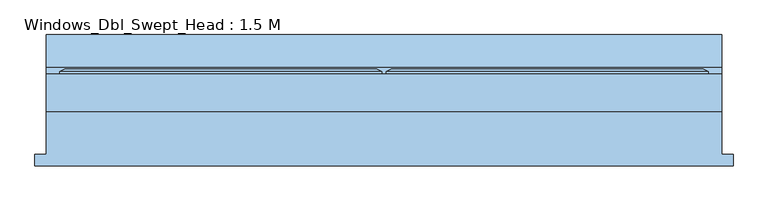
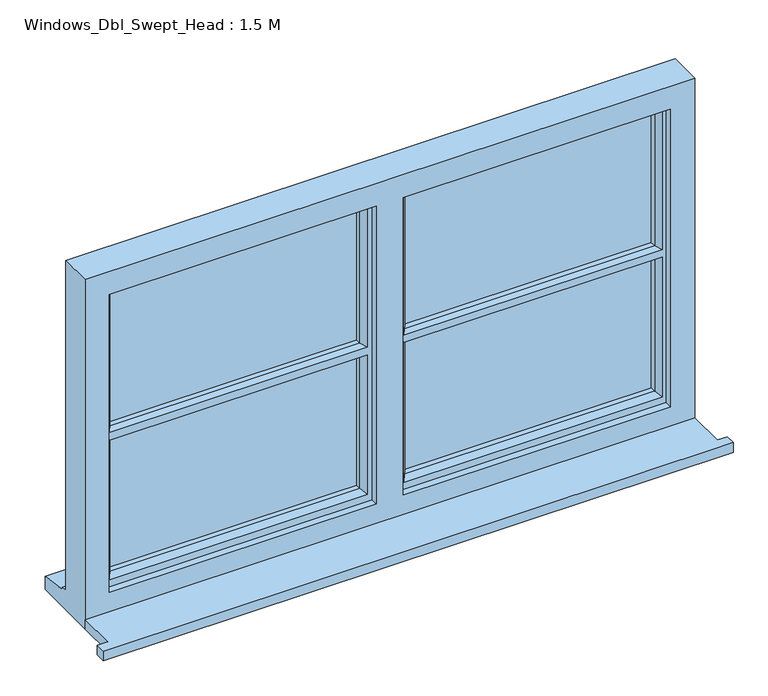
"""IFC4 building model written with IfcOpenShell, lengths in millimetres: window geometry, Windows_Dbl_Swept_Head : 1.5 M."""

from ifc_helpers import new_model, si_unit, frame, origin, place, context, project, spatial, polyline, circle_curve, outline, extrude, faceted_brep, source, transform, mapped, element, save
from ifc_brep_helpers import plane_surface, revolved_surface, advanced_brep


def windows_dbl_swept_head_1_5_m_7eee1f0c(model_context):
    return source(origin(), model_context, "Body", "SolidModel", [
        extrude(outline(polyline([(-1060.0, -130.8434322), (-1060.0, -105.8434322), (-1035.0, -105.8434322), (-1035.0, -10.2434322), (465.0, -10.2434322), (465.0, -105.8434322), (490.0, -105.8434322), (490.0, -130.8434322), (-1060.0, -130.8434322)])), frame((0.0, 0.0, 1200.0), z_axis=(0.0, 0.0, 1.0), x_axis=(1.0, 0.0, 0.0)), (0.0, 0.0, 1.0), 25.0),
        extrude(outline(polyline([(395.1480377, 36.7565678), (-240.0, 36.7565678), (-240.0, 60.7565678), (395.1480377, 60.7565678), (395.1480377, 36.7565678)])), frame((0.0, 0.0, 1293.0), z_axis=(0.0, 0.0, 1.0), x_axis=(1.0, 0.0, 0.0)), (0.0, 0.0, 1.0), 365.5),
        extrude(outline(polyline([(395.1480377, 36.7565678), (-240.0, 36.7565678), (-240.0, 60.7565678), (395.1480377, 60.7565678), (395.1480377, 36.7565678)])), frame((0.0, 0.0, 1674.5), z_axis=(0.0, 0.0, 1.0), x_axis=(1.0, 0.0, 0.0)), (0.0, 0.0, 1.0), 365.5),
        extrude(outline(polyline([(-330.0, 36.7565678), (-965.0, 36.7565678), (-965.0, 60.7565678), (-330.0, 60.7565678), (-330.0, 36.7565678)])), frame((0.0, 0.0, 1674.5), z_axis=(0.0, 0.0, 1.0), x_axis=(1.0, 0.0, 0.0)), (0.0, 0.0, 1.0), 365.5),
        extrude(outline(polyline([(-330.0, 36.7565678), (-965.1480377, 36.7565678), (-965.1480377, 60.7565678), (-330.0, 60.7565678), (-330.0, 36.7565678)])), frame((0.0, 0.0, 1292.8519623), z_axis=(0.0, 0.0, 1.0), x_axis=(1.0, 0.0, 0.0)), (0.0, 0.0, 1.0), 365.6480377),
        faceted_brep([(-1035.0, -10.2434322, 1200.0), (465.0, -10.2434322, 1200.0), (465.0, -10.2434322, 2110.0), (-1035.0, -10.2434322, 2110.0), (-318.0, -10.2434322, 2050.0), (-318.0, -10.2434322, 1275.0), (-975.0, -10.2434322, 1275.0), (-975.0, -10.2434322, 2050.0), (-252.0, -10.2434322, 2050.0), (405.0, -10.2434322, 2050.0), (405.0, -10.2434322, 1275.0), (-252.0, -10.2434322, 1275.0), (-1035.0, 72.7565678, 2110.0), (-1035.0, 72.7565678, 1251.0), (-1035.0, 87.7565678, 1249.68767), (-1035.0, 87.7565678, 1244.7449676), (-1035.0, 160.2565678, 1233.8088847), (-1035.0, 160.2565678, 1200.0), (465.0, 72.7565678, 2110.0), (465.0, 72.7565678, 1251.0), (-995.0, 72.7565678, 2070.0), (-995.0, 72.7565678, 1263.0), (-300.0, 72.7565678, 1263.0), (-300.0, 72.7565678, 2070.0), (-270.0, 72.7565678, 2070.0), (-270.0, 72.7565678, 1263.0), (425.0, 72.7565678, 1263.0), (425.0, 72.7565678, 2070.0), (-995.0, 7.7565678, 2070.0), (-995.0, 7.7565678, 1263.0), (-300.0, 7.7565678, 2070.0), (-300.0, 7.7565678, 1263.0), (-318.0, 7.7565678, 2050.0), (-975.0, 7.7565678, 2050.0), (-975.0, 7.7565678, 1275.0), (-318.0, 7.7565678, 1275.0), (-270.0, 7.7565678, 2070.0), (425.0, 7.7565678, 2070.0), (425.0, 7.7565678, 1263.0), (-270.0, 7.7565678, 1263.0), (405.0, 7.7565678, 2050.0), (-252.0, 7.7565678, 2050.0), (-252.0, 7.7565678, 1275.0), (405.0, 7.7565678, 1275.0), (465.0, 160.2565678, 1200.0), (465.0, 160.2565678, 1233.8088847), (465.0, 87.7565678, 1244.7449676), (465.0, 87.7565678, 1249.68767)], [[[0, 1, 2, 3], [4, 5, 6, 7], [8, 9, 10, 11]], [[0, 3, 12, 13, 14, 15, 16, 17]], [[13, 12, 18, 19], [20, 21, 22, 23], [24, 25, 26, 27]], [[21, 20, 28, 29]], [[28, 30, 31, 29], [32, 33, 34, 35]], [[36, 37, 38, 39], [40, 41, 42, 43]], [[33, 7, 6, 34]], [[12, 3, 2, 18]], [[28, 20, 23, 30]], [[27, 37, 36, 24]], [[7, 33, 32, 4]], [[40, 9, 8, 41]], [[19, 18, 2, 1, 44, 45, 46, 47]], [[27, 26, 38, 37]], [[9, 40, 43, 10]], [[23, 22, 31, 30]], [[25, 24, 36, 39]], [[41, 8, 11, 42]], [[4, 32, 35, 5]], [[44, 1, 0, 17]], [[45, 44, 17, 16]], [[46, 45, 16, 15]], [[47, 46, 15, 14]], [[19, 47, 14, 13]], [[22, 21, 29, 31]], [[26, 25, 39, 38]], [[11, 10, 43, 42]], [[35, 34, 6, 5]]]),
        advanced_brep(
        [(-280.0, 72.7565678, 2080.0), (-280.0, 78.5300705, 2080.0), (-280.0, 78.5300705, 1253.0), (-280.0, 72.7565678, 1253.0), (-270.0, 7.7565678, 2070.0), (-270.0, 72.7565678, 2070.0), (-270.0, 72.7565678, 1263.0), (-270.0, 7.7565678, 1263.0), (-230.0, 22.2494677, 2030.0), (-240.1480377, 7.7565678, 2040.1480377), (-240.1480377, 7.7565678, 1676.3519623), (-230.0, 22.2494677, 1681.5), (-240.1480377, 7.7565678, 1292.8519623), (-230.0, 22.2494677, 1303.0), (-230.0, 22.2494677, 1651.5), (-240.1480377, 7.7565678, 1656.6480377), (-230.0, 36.7565678, 2030.0), (-230.0, 36.7565678, 1681.5), (-230.0, 36.7565678, 1303.0), (-230.0, 36.7565678, 1651.5), (-240.0, 60.7565678, 2040.0), (-240.0, 36.7565678, 2040.0), (-240.0, 36.7565678, 1674.5), (-240.0, 60.7565678, 1674.5), (-240.0, 36.7565678, 1293.0), (-240.0, 60.7565678, 1293.0), (-240.0, 60.7565678, 1658.5), (-240.0, 36.7565678, 1658.5), (-230.0, 60.7565678, 1303.0), (-230.0, 78.5300705, 1303.0), (-230.0, 78.5300705, 1651.5), (-230.0, 60.7565678, 1651.5), (-230.0, 60.7565678, 1681.5), (-230.0, 78.5300705, 1681.5), (-230.0, 78.5300705, 1953.8431839), (-230.0, 60.7565678, 1953.8431839), (-247.4457548, 84.3035732, 2047.4457548), (-230.0, 78.5300705, 2030.0), (-235.0, 80.1847718, 1681.5), (-247.4457548, 84.3035732, 1669.0542452), (-247.4457548, 84.3035732, 1285.5542452), (-247.4457548, 84.3035732, 1663.9457548), (-235.0, 80.1847718, 1651.5), (-269.2153903, 84.3035732, 2069.2153903), (-269.2153903, 84.3035732, 1263.7846097), (435.0, 78.5300705, 1253.0), (435.0, 72.7565678, 1253.0), (425.0, 72.7565678, 1263.0), (425.0, 7.7565678, 1263.0), (395.1480377, 7.7565678, 1292.8519623), (385.0, 22.2494677, 1303.0), (385.0, 36.7565678, 1303.0), (395.0, 36.7565678, 1293.0), (395.0, 60.7565678, 1293.0), (385.0, 60.7565678, 1303.0), (385.0, 78.5300705, 1303.0), (402.4457548, 84.3035732, 1285.5542452), (424.2153903, 84.3035732, 1263.7846097), (435.0, 78.5300705, 2080.0), (435.0, 72.7565678, 2080.0), (425.0, 72.7565678, 2070.0), (425.0, 7.7565678, 2070.0), (395.1480377, 7.7565678, 1656.6480377), (385.0, 22.2494677, 1651.5), (395.1480377, 7.7565678, 2040.1480377), (385.0, 22.2494677, 2030.0), (385.0, 22.2494677, 1681.5), (395.1480377, 7.7565678, 1676.3519623), (385.0, 36.7565678, 1651.5), (385.0, 36.7565678, 2030.0), (385.0, 36.7565678, 1681.5), (395.0, 36.7565678, 1658.5), (395.0, 60.7565678, 1658.5), (395.0, 36.7565678, 2040.0), (395.0, 60.7565678, 2040.0), (395.0, 60.7565678, 1674.5), (395.0, 36.7565678, 1674.5), (385.0, 60.7565678, 1651.5), (385.0, 78.5300705, 1651.5), (385.0, 78.5300705, 1681.5), (385.0, 60.7565678, 1681.5), (385.0, 60.7565678, 1953.8431839), (385.0, 78.5300705, 1953.8431839), (390.0, 80.1847718, 1651.5), (402.4457548, 84.3035732, 1663.9457548), (385.0, 78.5300705, 2030.0), (402.4457548, 84.3035732, 2047.4457548), (402.4457548, 84.3035732, 1669.0542452), (390.0, 80.1847718, 1681.5), (424.2153903, 84.3035732, 2069.2153903)],
        [
            (0, 1),
            (1, 2),
            (2, 3),
            (3, 0),
            (4, 5),
            (5, 6),
            (6, 7),
            (7, 4),
            (8, 9),
            (9, 10),
            (10, 11),
            (11, 8),
            (12, 13),
            (13, 14),
            (14, 15),
            (15, 12),
            (16, 8),
            (11, 17),
            (17, 16),
            (13, 18),
            (18, 19),
            (19, 14),
            (20, 21),
            (21, 22),
            (22, 23),
            (23, 20),
            (24, 25),
            (25, 26),
            (26, 27),
            (27, 24),
            (28, 29),
            (29, 30),
            (30, 31),
            (31, 28),
            (32, 33),
            (33, 34),
            (34, 35),
            (35, 32),
            (36, 37),
            (37, 34),
            (33, 38),
            (38, 39),
            (39, 36),
            (29, 40),
            (40, 41),
            (41, 42),
            (42, 30),
            (1, 43),
            (43, 44),
            (44, 2),
            (2, 45),
            (45, 46),
            (46, 3),
            (6, 47),
            (47, 48),
            (48, 7),
            (12, 49),
            (49, 50),
            (50, 13),
            (50, 51),
            (51, 18),
            (24, 52),
            (52, 53),
            (53, 25),
            (28, 54),
            (54, 55),
            (55, 29),
            (55, 56),
            (56, 40),
            (44, 57),
            (57, 45),
            (45, 58),
            (58, 59),
            (59, 46),
            (47, 60),
            (60, 61),
            (61, 48),
            (49, 62),
            (62, 63),
            (63, 50),
            (64, 65),
            (65, 66),
            (66, 67),
            (67, 64),
            (63, 68),
            (68, 51),
            (65, 69),
            (69, 70),
            (70, 66),
            (52, 71),
            (71, 72),
            (72, 53),
            (73, 74),
            (74, 75),
            (75, 76),
            (76, 73),
            (54, 77),
            (77, 78),
            (78, 55),
            (79, 80),
            (80, 81),
            (81, 82),
            (82, 79),
            (78, 83),
            (83, 84),
            (84, 56),
            (85, 86),
            (86, 87),
            (87, 88),
            (88, 79),
            (82, 85),
            (57, 89),
            (89, 58),
            (0, 59),
            (58, 1),
            (5, 60),
            (4, 61),
            (15, 62),
            (9, 64),
            (67, 10),
            (8, 65),
            (16, 69),
            (27, 71),
            (68, 19),
            (21, 73),
            (76, 22),
            (17, 70),
            (20, 74),
            (72, 26),
            (31, 77),
            (23, 75),
            (80, 32),
            (35, 81, circle_curve(frame((77.5, 60.7565678, 1325.0), z_axis=(0.0, 1.0, 0.0), x_axis=(1.0, 0.0, 0.0)), 700.0)),
            (36, 86),
            (85, 37),
            (43, 89),
            (84, 41),
            (39, 87),
            (38, 88),
            (11, 66),
            (14, 63),
            (42, 83),
            (82, 34, circle_curve(frame((77.5, 78.5300705, 1325.0), z_axis=(0.0, -1.0, 0.0), x_axis=(1.0, 0.0, 0.0)), 700.0)),
        ],
        [
            plane_surface(frame((-280.0, 78.5300705, 2080.0), z_axis=(-1.0, 0.0, 0.0), x_axis=(0.0, 0.0, -1.0))),
            plane_surface(frame((-270.0, 72.7565678, 2070.0), z_axis=(-1.0, 0.0, 0.0), x_axis=(0.0, 0.0, -1.0))),
            plane_surface(frame((-240.1480377, 7.7565678, 2040.1480377), z_axis=(0.8191520442889492, -0.5735764363511071, 0.0), x_axis=(0.0, 0.0, -1.0))),
            plane_surface(frame((-230.0, 22.2494677, 2030.0), z_axis=(1.0, 0.0, 0.0), x_axis=(0.0, 0.0, -1.0))),
            plane_surface(frame((-240.0, 36.7565678, 2040.0), z_axis=(1.0, 0.0, 0.0), x_axis=(0.0, 0.0, -1.0))),
            plane_surface(frame((-230.0, 60.7565678, 2030.0), z_axis=(1.0, 0.0, 0.0), x_axis=(0.0, 0.0, -1.0))),
            plane_surface(frame((-230.0, 78.5300705, 2030.0), z_axis=(0.31418232948755237, 0.9493626619147053, 0.0), x_axis=(0.0, 0.0, -1.0))),
            plane_surface(frame((-269.2153903, 84.3035732, 2069.2153903), z_axis=(-0.47196942945730275, 0.8816149146071363, 0.0), x_axis=(0.0, 0.0, -1.0))),
            plane_surface(frame((-280.0, 78.5300705, 1253.0), z_axis=(0.0, 0.0, -1.0), x_axis=(1.0, 0.0, 0.0))),
            plane_surface(frame((-270.0, 72.7565678, 1263.0), z_axis=(0.0, 0.0, -1.0), x_axis=(1.0, 0.0, 0.0))),
            plane_surface(frame((-240.1480377, 7.7565678, 1292.8519623), z_axis=(0.0, -0.5735764363511044, 0.819152044288951), x_axis=(1.0, 0.0, 0.0))),
            plane_surface(frame((-230.0, 22.2494677, 1303.0), z_axis=(0.0, 0.0, 1.0), x_axis=(1.0, 0.0, 0.0))),
            plane_surface(frame((-240.0, 36.7565678, 1293.0), z_axis=(0.0, 0.0, 1.0), x_axis=(1.0, 0.0, 0.0))),
            plane_surface(frame((-230.0, 60.7565678, 1303.0), z_axis=(0.0, 0.0, 1.0), x_axis=(1.0, 0.0, 0.0))),
            plane_surface(frame((-230.0, 78.5300705, 1303.0), z_axis=(0.0, 0.9493626619147063, 0.31418232948754926), x_axis=(1.0, 0.0, 0.0))),
            plane_surface(frame((-269.2153903, 84.3035732, 1263.7846097), z_axis=(0.0, 0.8816149146071347, -0.47196942945730563), x_axis=(1.0, 0.0, 0.0))),
            plane_surface(frame((435.0, 78.5300705, 1253.0), z_axis=(1.0, 0.0, 0.0), x_axis=(0.0, 0.0, 1.0))),
            plane_surface(frame((425.0, 72.7565678, 1263.0), z_axis=(1.0, 0.0, 0.0), x_axis=(0.0, 0.0, 1.0))),
            plane_surface(frame((395.1480377, 7.7565678, 1292.8519623), z_axis=(-0.8191520442889529, -0.5735764363511018, 0.0), x_axis=(0.0, 0.0, 1.0))),
            plane_surface(frame((385.0, 22.2494677, 1303.0), z_axis=(-1.0, 0.0, 0.0), x_axis=(0.0, 0.0, 1.0))),
            plane_surface(frame((395.0, 36.7565678, 1293.0), z_axis=(-1.0, 0.0, 0.0), x_axis=(0.0, 0.0, 1.0))),
            plane_surface(frame((385.0, 60.7565678, 1303.0), z_axis=(-1.0, 0.0, 0.0), x_axis=(0.0, 0.0, 1.0))),
            plane_surface(frame((385.0, 78.5300705, 1303.0), z_axis=(-0.3141823294875462, 0.9493626619147074, 0.0), x_axis=(0.0, 0.0, 1.0))),
            plane_surface(frame((424.2153903, 84.3035732, 1263.7846097), z_axis=(0.4719694294573085, 0.8816149146071331, 0.0), x_axis=(0.0, 0.0, 1.0))),
            plane_surface(frame((435.0, 78.5300705, 2080.0), z_axis=(0.0, 0.0, 1.0), x_axis=(-1.0, 0.0, 0.0))),
            plane_surface(frame((435.0, 72.7565678, 2080.0), z_axis=(0.0, -1.0, 0.0), x_axis=(-1.0, 0.0, 0.0))),
            plane_surface(frame((425.0, 72.7565678, 2070.0), z_axis=(0.0, 0.0, 1.0), x_axis=(-1.0, 0.0, 0.0))),
            plane_surface(frame((425.0, 7.7565678, 2070.0), z_axis=(0.0, -1.0, 0.0), x_axis=(-1.0, 0.0, 0.0))),
            plane_surface(frame((395.1480377, 7.7565678, 2040.1480377), z_axis=(0.0, -0.5735764363511044, -0.819152044288951), x_axis=(-1.0, 0.0, 0.0))),
            plane_surface(frame((385.0, 22.2494677, 2030.0), z_axis=(0.0, 0.0, -1.0), x_axis=(-1.0, 0.0, 0.0))),
            plane_surface(frame((385.0, 36.7565678, 2030.0), z_axis=(0.0, 1.0, 0.0), x_axis=(-1.0, 0.0, 0.0))),
            plane_surface(frame((395.0, 36.7565678, 2040.0), z_axis=(0.0, 0.0, -1.0), x_axis=(-1.0, 0.0, 0.0))),
            plane_surface(frame((395.0, 60.7565678, 2040.0), z_axis=(0.0, -1.0, 0.0), x_axis=(-1.0, 0.0, 0.0))),
            plane_surface(frame((385.0, 78.5300705, 2030.0), z_axis=(0.0, 0.9493626619147064, -0.3141823294875493), x_axis=(-1.0, 0.0, 0.0))),
            plane_surface(frame((402.4457548, 84.3035732, 2047.4457548), z_axis=(0.0, 1.0, 0.0), x_axis=(-1.0, 0.0, 0.0))),
            plane_surface(frame((424.2153903, 84.3035732, 2069.2153903), z_axis=(0.0, 0.8816149146071347, 0.47196942945730563), x_axis=(-1.0, 0.0, 0.0))),
            plane_surface(frame((402.4457548, 84.3035732, 1669.0542452), z_axis=(0.0, 0.9493626619145938, 0.3141823294878896), x_axis=(-1.0, 0.0, 0.0))),
            plane_surface(frame((402.4457548, 80.1847718, 1681.5), z_axis=(0.0, 0.0, 1.0), x_axis=(-1.0, 0.0, 0.0))),
            plane_surface(frame((402.4457548, 60.7565678, 1674.5), z_axis=(0.0, 0.0, 1.0), x_axis=(-1.0, 0.0, 0.0))),
            plane_surface(frame((402.4457548, 36.7565678, 1681.5), z_axis=(0.0, 0.0, 1.0), x_axis=(-1.0, 0.0, 0.0))),
            plane_surface(frame((402.4457548, 22.2494677, 1681.5), z_axis=(0.0, -0.33472142672711697, 0.9423171262848634), x_axis=(-1.0, 0.0, 0.0))),
            plane_surface(frame((402.4457548, 7.7565678, 1656.6480377), z_axis=(0.0, -0.33472142672499106, -0.9423171262856186), x_axis=(-1.0, 0.0, 0.0))),
            plane_surface(frame((402.4457548, 22.2494677, 1651.5), z_axis=(0.0, 0.0, -1.0), x_axis=(-1.0, 0.0, 0.0))),
            plane_surface(frame((402.4457548, 36.7565678, 1658.5), z_axis=(0.0, 0.0, -1.0), x_axis=(-1.0, 0.0, 0.0))),
            plane_surface(frame((402.4457548, 60.7565678, 1651.5), z_axis=(0.0, 0.0, -1.0), x_axis=(-1.0, 0.0, 0.0))),
            plane_surface(frame((402.4457548, 80.1847718, 1651.5), z_axis=(0.0, 0.9493626619148547, -0.31418232948710106), x_axis=(-1.0, 0.0, 0.0))),
            plane_surface(frame((-230.0, 78.5300705, 2030.0), z_axis=(0.0, 1.0, 0.0), x_axis=(0.0, 0.0, 1.0))),
            revolved_surface(polyline([(777.5, 78.5300705, 1325.0), (777.5, 60.7565678, 1325.0)]), (77.5, 78.5300705, 1325.0), (0.0, 1.0, 0.0)),
        ],
        [
            (0, [[1, 2, 3, 4]]),
            (1, [[5, 6, 7, 8]]),
            (2, [[9, 10, 11, 12]]),
            (2, [[13, 14, 15, 16]]),
            (3, [[17, -12, 18, 19]]),
            (3, [[20, 21, 22, -14]]),
            (4, [[23, 24, 25, 26]]),
            (4, [[27, 28, 29, 30]]),
            (5, [[31, 32, 33, 34]]),
            (5, [[35, 36, 37, 38]]),
            (6, [[39, 40, -36, 41, 42, 43]]),
            (6, [[44, 45, 46, 47, -32]]),
            (7, [[-2, 48, 49, 50]]),
            (8, [[-3, 51, 52, 53]]),
            (9, [[-7, 54, 55, 56]]),
            (10, [[-13, 57, 58, 59]]),
            (11, [[-20, -59, 60, 61]]),
            (12, [[-27, 62, 63, 64]]),
            (13, [[-31, 65, 66, 67]]),
            (14, [[-44, -67, 68, 69]]),
            (15, [[-50, 70, 71, -51]]),
            (16, [[-52, 72, 73, 74]]),
            (17, [[-55, 75, 76, 77]]),
            (18, [[-58, 78, 79, 80]]),
            (18, [[81, 82, 83, 84]]),
            (19, [[-60, -80, 85, 86]]),
            (19, [[87, 88, 89, -82]]),
            (20, [[-63, 90, 91, 92]]),
            (20, [[93, 94, 95, 96]]),
            (21, [[-66, 97, 98, 99]]),
            (21, [[100, 101, 102, 103]]),
            (22, [[-68, -99, 104, 105, 106]]),
            (22, [[107, 108, 109, 110, -103, 111]]),
            (23, [[-71, 112, 113, -72]]),
            (24, [[-1, 114, -73, 115]]),
            (25, [[-4, -53, -74, -114], [-6, 116, -75, -54]]),
            (26, [[-5, 117, -76, -116]]),
            (27, [[-8, -56, -77, -117], [-57, -16, 118, -78], [119, -84, 120, -10]]),
            (28, [[-9, 121, -81, -119]]),
            (29, [[-17, 122, -87, -121]]),
            (30, [[-62, -30, 123, -90], [-61, -86, 124, -21]]),
            (30, [[125, -96, 126, -24], [-122, -19, 127, -88]]),
            (31, [[-23, 128, -93, -125]]),
            (32, [[-64, -92, 129, -28], [-65, -34, 130, -97]]),
            (32, [[-128, -26, 131, -94], [132, -38, 133, -101]]),
            (33, [[-39, 134, -107, 135]]),
            (34, [[-49, 136, -112, -70], [-69, -106, 137, -45], [-134, -43, 138, -108]]),
            (35, [[-48, -115, -113, -136]]),
            (36, [[-138, -42, 139, -109]]),
            (37, [[-132, -100, -110, -139, -41, -35]]),
            (38, [[-25, -126, -95, -131]]),
            (39, [[140, -89, -127, -18]]),
            (40, [[-120, -83, -140, -11]]),
            (41, [[-118, -15, 141, -79]]),
            (42, [[-141, -22, -124, -85]]),
            (43, [[-29, -129, -91, -123]]),
            (44, [[-130, -33, -47, 142, -104, -98]]),
            (45, [[-137, -105, -142, -46]]),
            (46, [[143, -40, -135, -111]]),
            (47, [[-133, -37, -143, -102]]),
        ],
    ),
        advanced_brep(
        [(-330.0, 60.7565678, 2040.0), (-965.0, 60.7565678, 2040.0), (-965.0, 60.7565678, 1674.5), (-330.0, 60.7565678, 1674.5), (-955.0, 60.7565678, 1953.8431839), (-340.0, 60.7565678, 1953.8431839), (-340.0, 60.7565678, 1681.5), (-955.0, 60.7565678, 1681.5), (-965.0, 60.7565678, 1293.0), (-330.0, 60.7565678, 1293.0), (-330.0, 60.7565678, 1658.5), (-965.0, 60.7565678, 1658.5), (-340.0, 60.7565678, 1303.0), (-955.0, 60.7565678, 1303.0), (-955.0, 60.7565678, 1651.5), (-340.0, 60.7565678, 1651.5), (-1005.0, 72.7565678, 2080.0), (-1005.0, 78.5300705, 2080.0), (-1005.0, 78.5300705, 1253.0), (-1005.0, 72.7565678, 1253.0), (-995.0, 7.7565678, 2070.0), (-995.0, 72.7565678, 2070.0), (-995.0, 72.7565678, 1263.0), (-995.0, 7.7565678, 1263.0), (-955.0, 22.2494677, 2030.0), (-965.1480377, 7.7565678, 2040.1480377), (-965.1480377, 7.7565678, 1676.3519623), (-955.0, 22.2494677, 1681.5), (-965.1480377, 7.7565678, 1292.8519623), (-955.0, 22.2494677, 1303.0), (-955.0, 22.2494677, 1651.5), (-965.1480377, 7.7565678, 1656.6480377), (-955.0, 36.7565678, 2030.0), (-955.0, 36.7565678, 1681.5), (-955.0, 36.7565678, 1303.0), (-955.0, 36.7565678, 1651.5), (-965.0, 36.7565678, 2040.0), (-965.0, 36.7565678, 1674.5), (-965.0, 36.7565678, 1293.0), (-965.0, 36.7565678, 1658.5), (-955.0, 78.5300705, 1303.0), (-955.0, 78.5300705, 1651.5), (-955.0, 78.5300705, 1681.5), (-955.0, 78.5300705, 1953.8431839), (-972.4457548, 84.3035732, 2047.4457548), (-955.0, 78.5300705, 2030.0), (-960.0, 80.1847718, 1681.5), (-972.4457548, 84.3035732, 1669.0542452), (-972.4457548, 84.3035732, 1285.5542452), (-972.4457548, 84.3035732, 1663.9457548), (-960.0, 80.1847718, 1651.5), (-994.2153903, 84.3035732, 2069.2153903), (-994.2153903, 84.3035732, 1263.7846097), (-290.0, 78.5300705, 1253.0), (-290.0, 72.7565678, 1253.0), (-300.0, 72.7565678, 1263.0), (-300.0, 7.7565678, 1263.0), (-329.8519623, 7.7565678, 1292.8519623), (-340.0, 22.2494677, 1303.0), (-340.0, 36.7565678, 1303.0), (-330.0, 36.7565678, 1293.0), (-340.0, 78.5300705, 1303.0), (-322.5542452, 84.3035732, 1285.5542452), (-300.7846097, 84.3035732, 1263.7846097), (-290.0, 78.5300705, 2080.0), (-290.0, 72.7565678, 2080.0), (-300.0, 72.7565678, 2070.0), (-300.0, 7.7565678, 2070.0), (-329.8519623, 7.7565678, 1656.6480377), (-340.0, 22.2494677, 1651.5), (-329.8519623, 7.7565678, 2040.1480377), (-340.0, 22.2494677, 2030.0), (-340.0, 22.2494677, 1681.5), (-329.8519623, 7.7565678, 1676.3519623), (-340.0, 36.7565678, 1651.5), (-340.0, 36.7565678, 2030.0), (-340.0, 36.7565678, 1681.5), (-330.0, 36.7565678, 1658.5), (-330.0, 36.7565678, 2040.0), (-330.0, 36.7565678, 1674.5), (-340.0, 78.5300705, 1651.5), (-340.0, 78.5300705, 1681.5), (-340.0, 78.5300705, 1953.8431839), (-335.0, 80.1847718, 1651.5), (-322.5542452, 84.3035732, 1663.9457548), (-340.0, 78.5300705, 2030.0), (-322.5542452, 84.3035732, 2047.4457548), (-322.5542452, 84.3035732, 1669.0542452), (-335.0, 80.1847718, 1681.5), (-300.7846097, 84.3035732, 2069.2153903)],
        [
            (0, 1),
            (1, 2),
            (2, 3),
            (3, 0),
            (4, 5, circle_curve(frame((-647.5, 60.7565678, 1325.0), z_axis=(0.0, 1.0, 0.0), x_axis=(1.0, 0.0, 0.0)), 700.0)),
            (5, 6),
            (6, 7),
            (7, 4),
            (8, 9),
            (9, 10),
            (10, 11),
            (11, 8),
            (12, 13),
            (13, 14),
            (14, 15),
            (15, 12),
            (16, 17),
            (17, 18),
            (18, 19),
            (19, 16),
            (20, 21),
            (21, 22),
            (22, 23),
            (23, 20),
            (24, 25),
            (25, 26),
            (26, 27),
            (27, 24),
            (28, 29),
            (29, 30),
            (30, 31),
            (31, 28),
            (32, 24),
            (27, 33),
            (33, 32),
            (29, 34),
            (34, 35),
            (35, 30),
            (1, 36),
            (36, 37),
            (37, 2),
            (38, 8),
            (11, 39),
            (39, 38),
            (13, 40),
            (40, 41),
            (41, 14),
            (7, 42),
            (42, 43),
            (43, 4),
            (44, 45),
            (45, 43),
            (42, 46),
            (46, 47),
            (47, 44),
            (40, 48),
            (48, 49),
            (49, 50),
            (50, 41),
            (17, 51),
            (51, 52),
            (52, 18),
            (18, 53),
            (53, 54),
            (54, 19),
            (22, 55),
            (55, 56),
            (56, 23),
            (28, 57),
            (57, 58),
            (58, 29),
            (58, 59),
            (59, 34),
            (38, 60),
            (60, 9),
            (12, 61),
            (61, 40),
            (61, 62),
            (62, 48),
            (52, 63),
            (63, 53),
            (53, 64),
            (64, 65),
            (65, 54),
            (55, 66),
            (66, 67),
            (67, 56),
            (57, 68),
            (68, 69),
            (69, 58),
            (70, 71),
            (71, 72),
            (72, 73),
            (73, 70),
            (69, 74),
            (74, 59),
            (71, 75),
            (75, 76),
            (76, 72),
            (60, 77),
            (77, 10),
            (78, 0),
            (3, 79),
            (79, 78),
            (15, 80),
            (80, 61),
            (81, 6),
            (5, 82),
            (82, 81),
            (80, 83),
            (83, 84),
            (84, 62),
            (85, 86),
            (86, 87),
            (87, 88),
            (88, 81),
            (82, 85),
            (63, 89),
            (89, 64),
            (16, 65),
            (64, 17),
            (21, 66),
            (20, 67),
            (31, 68),
            (25, 70),
            (73, 26),
            (24, 71),
            (32, 75),
            (39, 77),
            (74, 35),
            (36, 78),
            (79, 37),
            (33, 76),
            (44, 86),
            (85, 45),
            (51, 89),
            (84, 49),
            (47, 87),
            (46, 88),
            (83, 50),
            (69, 30),
            (72, 27),
            (82, 43, circle_curve(frame((-647.5, 78.5300705, 1325.0), z_axis=(0.0, -1.0, 0.0), x_axis=(1.0, 0.0, 0.0)), 700.0)),
        ],
        [
            plane_surface(frame((395.0, 60.7565678, 2040.0), z_axis=(0.0, -1.0, 0.0), x_axis=(-1.0, 0.0, 0.0))),
            plane_surface(frame((-1005.0, 78.5300705, 2080.0), z_axis=(-1.0, 0.0, 0.0), x_axis=(0.0, 0.0, -1.0))),
            plane_surface(frame((-995.0, 72.7565678, 2070.0), z_axis=(-1.0, 0.0, 0.0), x_axis=(0.0, 0.0, -1.0))),
            plane_surface(frame((-965.1480377, 7.7565678, 2040.1480377), z_axis=(0.8191520442889492, -0.5735764363511071, 0.0), x_axis=(0.0, 0.0, -1.0))),
            plane_surface(frame((-955.0, 22.2494677, 2030.0), z_axis=(1.0, 0.0, 0.0), x_axis=(0.0, 0.0, -1.0))),
            plane_surface(frame((-965.0, 36.7565678, 2040.0), z_axis=(1.0, 0.0, 0.0), x_axis=(0.0, 0.0, -1.0))),
            plane_surface(frame((-955.0, 60.7565678, 2030.0), z_axis=(1.0, 0.0, 0.0), x_axis=(0.0, 0.0, -1.0))),
            plane_surface(frame((-955.0, 78.5300705, 2030.0), z_axis=(0.31418232948755237, 0.9493626619147053, 0.0), x_axis=(0.0, 0.0, -1.0))),
            plane_surface(frame((-994.2153903, 84.3035732, 2069.2153903), z_axis=(-0.47196942945730275, 0.8816149146071363, 0.0), x_axis=(0.0, 0.0, -1.0))),
            plane_surface(frame((-1005.0, 78.5300705, 1253.0), z_axis=(0.0, 0.0, -1.0), x_axis=(1.0, 0.0, 0.0))),
            plane_surface(frame((-995.0, 72.7565678, 1263.0), z_axis=(0.0, 0.0, -1.0), x_axis=(1.0, 0.0, 0.0))),
            plane_surface(frame((-965.1480377, 7.7565678, 1292.8519623), z_axis=(0.0, -0.5735764363511044, 0.819152044288951), x_axis=(1.0, 0.0, 0.0))),
            plane_surface(frame((-955.0, 22.2494677, 1303.0), z_axis=(0.0, 0.0, 1.0), x_axis=(1.0, 0.0, 0.0))),
            plane_surface(frame((-965.0, 36.7565678, 1293.0), z_axis=(0.0, 0.0, 1.0), x_axis=(1.0, 0.0, 0.0))),
            plane_surface(frame((-955.0, 60.7565678, 1303.0), z_axis=(0.0, 0.0, 1.0), x_axis=(1.0, 0.0, 0.0))),
            plane_surface(frame((-955.0, 78.5300705, 1303.0), z_axis=(0.0, 0.9493626619147063, 0.31418232948754926), x_axis=(1.0, 0.0, 0.0))),
            plane_surface(frame((-994.2153903, 84.3035732, 1263.7846097), z_axis=(0.0, 0.8816149146071347, -0.47196942945730563), x_axis=(1.0, 0.0, 0.0))),
            plane_surface(frame((-290.0, 78.5300705, 1253.0), z_axis=(1.0, 0.0, 0.0), x_axis=(0.0, 0.0, 1.0))),
            plane_surface(frame((-300.0, 72.7565678, 1263.0), z_axis=(1.0, 0.0, 0.0), x_axis=(0.0, 0.0, 1.0))),
            plane_surface(frame((-329.8519623, 7.7565678, 1292.8519623), z_axis=(-0.8191520442889529, -0.5735764363511018, 0.0), x_axis=(0.0, 0.0, 1.0))),
            plane_surface(frame((-340.0, 22.2494677, 1303.0), z_axis=(-1.0, 0.0, 0.0), x_axis=(0.0, 0.0, 1.0))),
            plane_surface(frame((-330.0, 36.7565678, 1293.0), z_axis=(-1.0, 0.0, 0.0), x_axis=(0.0, 0.0, 1.0))),
            plane_surface(frame((-340.0, 60.7565678, 1303.0), z_axis=(-1.0, 0.0, 0.0), x_axis=(0.0, 0.0, 1.0))),
            plane_surface(frame((-340.0, 78.5300705, 1303.0), z_axis=(-0.3141823294875462, 0.9493626619147074, 0.0), x_axis=(0.0, 0.0, 1.0))),
            plane_surface(frame((-300.7846097, 84.3035732, 1263.7846097), z_axis=(0.4719694294573085, 0.8816149146071331, 0.0), x_axis=(0.0, 0.0, 1.0))),
            plane_surface(frame((-290.0, 78.5300705, 2080.0), z_axis=(0.0, 0.0, 1.0), x_axis=(-1.0, 0.0, 0.0))),
            plane_surface(frame((-290.0, 72.7565678, 2080.0), z_axis=(0.0, -1.0, 0.0), x_axis=(-1.0, 0.0, 0.0))),
            plane_surface(frame((-300.0, 72.7565678, 2070.0), z_axis=(0.0, 0.0, 1.0), x_axis=(-1.0, 0.0, 0.0))),
            plane_surface(frame((-300.0, 7.7565678, 2070.0), z_axis=(0.0, -1.0, 0.0), x_axis=(-1.0, 0.0, 0.0))),
            plane_surface(frame((-329.8519623, 7.7565678, 2040.1480377), z_axis=(0.0, -0.5735764363511044, -0.819152044288951), x_axis=(-1.0, 0.0, 0.0))),
            plane_surface(frame((-340.0, 22.2494677, 2030.0), z_axis=(0.0, 0.0, -1.0), x_axis=(-1.0, 0.0, 0.0))),
            plane_surface(frame((-340.0, 36.7565678, 2030.0), z_axis=(0.0, 1.0, 0.0), x_axis=(-1.0, 0.0, 0.0))),
            plane_surface(frame((-330.0, 36.7565678, 2040.0), z_axis=(0.0, 0.0, -1.0), x_axis=(-1.0, 0.0, 0.0))),
            plane_surface(frame((-340.0, 78.5300705, 2030.0), z_axis=(0.0, 0.9493626619147064, -0.3141823294875493), x_axis=(-1.0, 0.0, 0.0))),
            plane_surface(frame((-322.5542452, 84.3035732, 2047.4457548), z_axis=(0.0, 1.0, 0.0), x_axis=(-1.0, 0.0, 0.0))),
            plane_surface(frame((-300.7846097, 84.3035732, 2069.2153903), z_axis=(0.0, 0.8816149146071347, 0.47196942945730563), x_axis=(-1.0, 0.0, 0.0))),
            plane_surface(frame((-972.4457548, 80.1847718, 1681.5), z_axis=(0.0, 0.9493626619144715, 0.31418232948825914), x_axis=(1.0, 0.0, 0.0))),
            plane_surface(frame((-972.4457548, 84.3035732, 1663.9457548), z_axis=(0.0, 0.949362661914977, -0.3141823294867314), x_axis=(1.0, 0.0, 0.0))),
            plane_surface(frame((-972.4457548, 80.1847718, 1651.5), z_axis=(0.0, 0.0, -1.0), x_axis=(1.0, 0.0, 0.0))),
            plane_surface(frame((-972.4457548, 60.7565678, 1658.5), z_axis=(0.0, 0.0, -1.0), x_axis=(1.0, 0.0, 0.0))),
            plane_surface(frame((-972.4457548, 36.7565678, 1651.5), z_axis=(0.0, 0.0, -1.0), x_axis=(1.0, 0.0, 0.0))),
            plane_surface(frame((-972.4457548, 22.2494677, 1651.5), z_axis=(0.0, -0.3347214267259168, -0.9423171262852897), x_axis=(1.0, 0.0, 0.0))),
            plane_surface(frame((-972.4457548, 7.7565678, 1676.3519623), z_axis=(0.0, -0.33472142672616695, 0.9423171262852009), x_axis=(1.0, 0.0, 0.0))),
            plane_surface(frame((-972.4457548, 22.2494677, 1681.5), z_axis=(0.0, 0.0, 1.0), x_axis=(1.0, 0.0, 0.0))),
            plane_surface(frame((-972.4457548, 36.7565678, 1674.5), z_axis=(0.0, 0.0, 1.0), x_axis=(1.0, 0.0, 0.0))),
            plane_surface(frame((-972.4457548, 60.7565678, 1681.5), z_axis=(0.0, 0.0, 1.0), x_axis=(1.0, 0.0, 0.0))),
            plane_surface(frame((-230.0, 78.5300705, 2030.0), z_axis=(0.0, 1.0, 0.0), x_axis=(0.0, 0.0, 1.0))),
            revolved_surface(polyline([(52.5, 78.5300705, 1325.0), (52.5, 60.7565678, 1325.0)]), (-647.5, 72.7565678, 1325.0), (0.0, 1.0, 0.0)),
        ],
        [
            (0, [[1, 2, 3, 4], [5, 6, 7, 8]]),
            (0, [[9, 10, 11, 12], [13, 14, 15, 16]]),
            (1, [[17, 18, 19, 20]]),
            (2, [[21, 22, 23, 24]]),
            (3, [[25, 26, 27, 28]]),
            (3, [[29, 30, 31, 32]]),
            (4, [[33, -28, 34, 35]]),
            (4, [[36, 37, 38, -30]]),
            (5, [[39, 40, 41, -2]]),
            (5, [[42, -12, 43, 44]]),
            (6, [[45, 46, 47, -14]]),
            (6, [[48, 49, 50, -8]]),
            (7, [[51, 52, -49, 53, 54, 55]]),
            (7, [[56, 57, 58, 59, -46]]),
            (8, [[-18, 60, 61, 62]]),
            (9, [[-19, 63, 64, 65]]),
            (10, [[-23, 66, 67, 68]]),
            (11, [[-29, 69, 70, 71]]),
            (12, [[-36, -71, 72, 73]]),
            (13, [[-42, 74, 75, -9]]),
            (14, [[-45, -13, 76, 77]]),
            (15, [[-56, -77, 78, 79]]),
            (16, [[-62, 80, 81, -63]]),
            (17, [[-64, 82, 83, 84]]),
            (18, [[-67, 85, 86, 87]]),
            (19, [[-70, 88, 89, 90]]),
            (19, [[91, 92, 93, 94]]),
            (20, [[-72, -90, 95, 96]]),
            (20, [[97, 98, 99, -92]]),
            (21, [[-75, 100, 101, -10]]),
            (21, [[102, -4, 103, 104]]),
            (22, [[-76, -16, 105, 106]]),
            (22, [[107, -6, 108, 109]]),
            (23, [[-78, -106, 110, 111, 112]]),
            (23, [[113, 114, 115, 116, -109, 117]]),
            (24, [[-81, 118, 119, -82]]),
            (25, [[-17, 120, -83, 121]]),
            (26, [[-20, -65, -84, -120], [-22, 122, -85, -66]]),
            (27, [[-21, 123, -86, -122]]),
            (28, [[-24, -68, -87, -123], [-69, -32, 124, -88], [125, -94, 126, -26]]),
            (29, [[-25, 127, -91, -125]]),
            (30, [[-33, 128, -97, -127]]),
            (31, [[-74, -44, 129, -100], [-73, -96, 130, -37]]),
            (31, [[131, -104, 132, -40], [-128, -35, 133, -98]]),
            (32, [[-39, -1, -102, -131]]),
            (33, [[-51, 134, -113, 135]]),
            (34, [[-61, 136, -118, -80], [-79, -112, 137, -57], [-134, -55, 138, -114]]),
            (35, [[-60, -121, -119, -136]]),
            (36, [[-138, -54, 139, -115]]),
            (37, [[-137, -111, 140, -58]]),
            (38, [[-15, -47, -59, -140, -110, -105]]),
            (39, [[-43, -11, -101, -129]]),
            (40, [[141, -38, -130, -95]]),
            (41, [[-124, -31, -141, -89]]),
            (42, [[-126, -93, 142, -27]]),
            (43, [[-142, -99, -133, -34]]),
            (44, [[-41, -132, -103, -3]]),
            (45, [[-7, -107, -116, -139, -53, -48]]),
            (46, [[143, -52, -135, -117]]),
            (47, [[-5, -50, -143, -108]]),
        ],
    ),
    ])


if __name__ == "__main__":
    model = new_model("IFC4")
    model_context = context("Model", 3, world=origin())
    ifc_project = project(units=[si_unit("LENGTHUNIT", "METRE", prefix="MILLI")], contexts=[model_context])
    site = spatial("IfcSite", under=ifc_project)
    building = spatial("IfcBuilding", under=site)
    placement = place(None, origin())
    windows_dbl_swept_head_1_5_m_shape = windows_dbl_swept_head_1_5_m_7eee1f0c(model_context)
    element("IfcWindow", 1, ObjectType="Windows_Dbl_Swept_Head : 1.5 M", at=placement, inside=building, context=model_context, shape_type="MappedRepresentation", body=[
        mapped(windows_dbl_swept_head_1_5_m_shape, transform((0.0, 0.0, 0.0), x_axis=(1.0, 0.0, 0.0), y_axis=(0.0, 1.0, 0.0), z_axis=(0.0, 0.0, 1.0))),
    ])
    save(model, "model.ifc")

# Revit data of these elements
# Type "Windows_Dbl_Swept_Head : 1.5 M"
#   Type Mark = "70"
#   Operation = "DoublePanelVertical"
#   Construction Type Id = "GSP4R"
#   Manufacturer = "Revit"
#   Keynote = "L10"
#   Analytic Construction = "1/8 in Pilkington single glazing"
#   Wrap Layers (Ext) from Ext = 0.1025 m
#   Wrap Layers (Int) from Ext = 0.1775 m
#   Window Board Projection = 0.025 m
#   Window Board Extension = 0.025 m
#   Visual Light Transmittance = 0.9
#   Solar Heat Gain Coefficient = 0.78
#   Rough Width = 1.5 m
#   Rough Height = 0.91 m
#   Radius - Swept Head = 0.7 m
#   Height = 0.91 m
#   Width = 1.5 m
#   Heat Transfer Coefficient (U) = 3.6886 W/(m²·K)
#   Glazing Thickness = 0.024 m
#   FrameOffset - External = 0.05 m
#   Frame Depth = 0.065 m
#   Default Head Height = 2.11 m
#   Cill Depth = 0.0875 m
#   Cavity Closer Width = 0.05 m
#   Cavity Closer Offset from Ext = 0.1025 m
#   Cavity Closer Depth = 0.085 m
#   Vis - Cavity Closers = yes
#   Define Thermal Properties by = 1
#   Material Trim = Window Frame
#   Material Glass = Glass
#   Material Frame = Window Frame
#   Wall Closure = (empty or 0)
# Element 1 (IfcWindow, "Windows_Dbl_Swept_Head : 1.5 M")
#   Materials on its faces: "Window Frame", "Glass"
# Materials
#   "Window Frame": colour RGB 249 249 249, transparency 0, Keynote = "L10", Cost = 0
#   "Glass": class "Glass", colour RGB 0 128 192, transparency 0.9, Description = "Soda Lime Glass", Cost = 0
